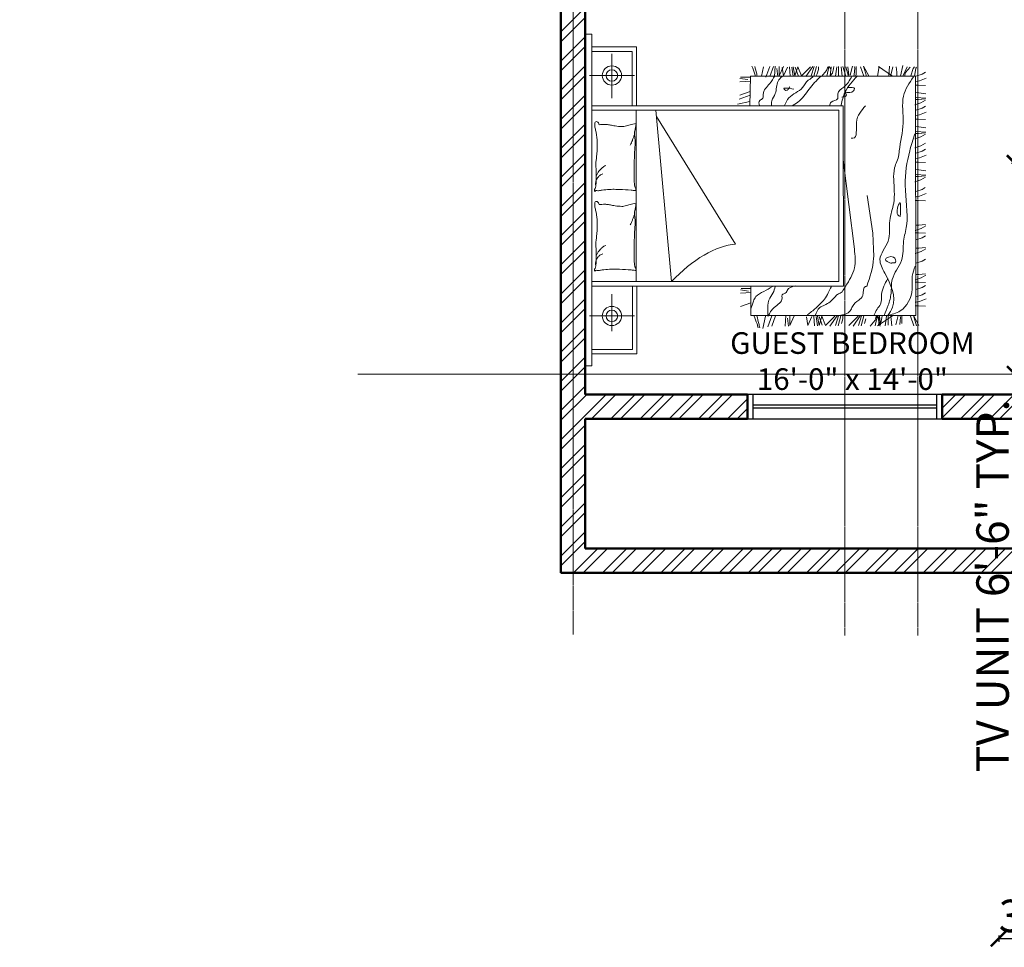
# Model space of a CAD drawing. Units: inches. Extents: x 261 to 2725, y 291 to 1454.
# Tile 17 of 35: x 1043 to 1407, y 301 to 644. Entities that reach past the tile are written whole.
import ezdxf

# ---------------------------------------------------------------- set-up
doc = ezdxf.new("R2010")
doc.units = ezdxf.units.IN
doc.linetypes.add('CENTER', pattern=[2, 1.25, -0.25, 0.25, -0.25])
for name, color, linetype, lineweight in [('A-ANNO-DIMS', 136, 'Continuous', 18), ('A-AREA-IDEN', 18, 'Continuous', 18), ('A-DOOR', 160, 'Continuous', 25), ('A-FURN', 30, 'Continuous', 18), ('A-GLAZ', 150, 'Continuous', 25), ('A-GRID', 251, 'CENTER', 13), ('A-WALL', 222, 'Continuous', 50), ('A-WALL-PATT', 243, 'Continuous', 13)]:
    doc.layers.add(name, color=color, linetype=linetype, lineweight=lineweight)
doc.styles.get("Standard").update_dxf_attribs({"font": 'arial.ttf'})
doc.dimstyles.new('ISO-25', dxfattribs={"dimtxt": 12, "dimasz": 6, "dimexe": 1.25, "dimexo": 0.625, "dimtad": 1, "dimdec": 0, "dimlunit": 3, "dimtxsty": 'Standard', "dimblk": 'ARCHTICK', "dimcen": 2.5, "dimadec": 0, "dimazin": 0, "dimtfac": 1, "dimtdec": 0, "dimtmove": 0, "dimatfit": 3, "dimfxl": 1, "dimfxlon": 1, "dimarcsym": 0})

# ---------------------------------------------------------------- blocks, each defined once
blk = doc.blocks.new('*U6')
for p, q in [((-36, 0), (-36, 6)), ((0, 0), (0, 6))]:
    blk.add_line(p, q)
blk.add_lwpolyline([(0, 0), (0, -36), (-1.75, -36), (-1.75, 0)], close=True)
blk.add_arc((0, 0), 36, 180, 270)
blk = doc.blocks.new('A$C2B723114')
for p, q in [((0, 2.9047), (2.8274, 2.9047)), ((0, 2.8487), (0, 2.9047)), ((0.4243, 2.8697), (0.4243, 2.4855)), ((2.4742, 2.8697), (2.4742, 2.4855)), ((2.8274, 2.9047), (2.8274, 2.8487)), ((2.8274, 2.8487), (0, 2.8487)), ((0.1012, 2.4649), (0.1012, 2.849)), ((0.1396, 2.5033), (0.1396, 2.849)), ((0.6794, 0.7051), (0.6794, 2.8509)), ((0.7187, 0.7435), (0.7187, 2.8509)), ((2.1776, 2.8509), (2.1776, 0.7454)), ((2.216, 2.8509), (2.216, 0.707)), ((2.6798, 2.5052), (2.6798, 2.8509)), ((2.7182, 2.4668), (2.7182, 2.8509)), ((0.6087, 2.6776), (0.295, 2.6776)), ((2.6586, 2.6776), (2.2821, 2.6776)), ((1.3789, 2.4999), (1.3598, 2.5761)), ((2.0593, 2.4999), (2.0402, 2.5761)), ((0.6794, 2.4649), (0.1012, 2.4649)), ((0.6766, 2.5033), (0.1396, 2.5033)), ((0.7191, 2.47), (2.1778, 2.4719)), ((1.3858, 2.4723), (1.3789, 2.4999)), ((2.0662, 2.4723), (2.0593, 2.4999)), ((2.2188, 2.5052), (2.6798, 2.5052)), ((2.2188, 2.4668), (2.7182, 2.4668)), ((2.1771, 2.3036), (0.718, 2.1685)), ((1.0365, 1.6233), (2.1246, 2.2989)), ((2.2287, 1.6076), (2.2523, 1.5035)), ((0.5047, 1.5819), (0.5353, 1.4945)), ((0.6174, 1.5819), (0.6232, 1.4916)), ((0.6467, 1.5819), (0.6369, 1.5137)), ((0.6571, 1.4945), (0.6571, 1.5765)), ((2.2726, 1.593), (2.3061, 1.5007)), ((2.3067, 1.5881), (2.3373, 1.5007)), ((2.4194, 1.5881), (2.4251, 1.4979)), ((2.4487, 1.5881), (2.4389, 1.5199)), ((2.4591, 1.5007), (2.4591, 1.5828)), ((0.4269, 0.0884), (0.4269, 1.4945)), ((0.4269, 1.4945), (0.6794, 1.4945)), ((2.4685, 1.4964), (2.216, 1.5022)), ((2.4685, 1.4964), (2.4685, 0.0903)), ((0.3172, 1.3923), (0.4213, 1.3687)), ((0.3318, 1.3485), (0.4241, 1.3149)), ((2.4596, 1.3659), (2.552, 1.3324)), ((2.4685, 1.4044), (2.5491, 1.3861)), ((0.3367, 1.3143), (0.4241, 1.2838)), ((2.4645, 1.3318), (2.552, 1.3012)), ((2.4645, 1.2928), (2.5548, 1.2871)), ((2.4645, 1.2635), (2.5328, 1.2733)), ((0.3367, 1.2016), (0.427, 1.1959)), ((0.3367, 1.1724), (0.405, 1.1821)), ((2.4699, 1.2531), (2.552, 1.2163)), ((2.552, 1.2531), (2.4699, 1.2531)), ((2.5435, 1.2276), (2.4699, 1.2163)), ((2.4699, 1.2163), (2.5463, 1.1823)), ((0.4241, 1.162), (0.3421, 1.162)), ((0.3421, 1.162), (0.4241, 1.1252)), ((2.5491, 1.1654), (2.467, 1.1597)), ((2.5463, 1.1455), (2.467, 1.1342)), ((2.5491, 1.1342), (2.4699, 1.1201)), ((2.4699, 1.1201), (2.5491, 1.0946)), ((2.5491, 1.0946), (2.4699, 1.0635)), ((2.5463, 1.1172), (2.4727, 1.0918)), ((0.4157, 1.0206), (0.3421, 1.0093)), ((0.3421, 1.0093), (0.4185, 0.9754)), ((2.4642, 1.0267), (2.552, 0.9644)), ((2.4699, 1.0635), (2.5491, 0.9842)), ((0.4213, 0.9584), (0.3392, 0.9527)), ((0.4185, 0.9386), (0.3392, 0.9272)), ((0.4213, 0.9272), (0.3421, 0.9131)), ((2.4642, 0.9389), (2.4869, 0.9276)), ((2.467, 0.9559), (2.552, 0.9333)), ((2.4699, 0.9785), (2.552, 0.9531)), ((2.4869, 0.9276), (2.5265, 0.9163)), ((0.3421, 0.9131), (0.4213, 0.8876)), ((0.4213, 0.8876), (0.3421, 0.8565)), ((0.3421, 0.8565), (0.4213, 0.7772)), ((0.4185, 0.9103), (0.3449, 0.8848)), ((2.4642, 0.8908), (2.5152, 0.8483)), ((2.467, 0.8455), (2.5208, 0.8342)), ((2.5152, 0.8483), (2.5491, 0.837)), ((2.5265, 0.9163), (2.5491, 0.9163)), ((0.3364, 0.8197), (0.4241, 0.7574)), ((0.3421, 0.7716), (0.4241, 0.7461)), ((2.5491, 0.7606), (2.467, 0.7719)), ((2.4699, 0.8172), (2.4925, 0.7974)), ((2.5491, 0.8087), (2.4699, 0.8172)), ((2.4925, 0.7974), (2.535, 0.7889)), ((2.5208, 0.8342), (2.552, 0.8285)), ((2.552, 0.8285), (2.5293, 0.8087)), ((2.535, 0.7889), (2.552, 0.7861)), ((0.3392, 0.7489), (0.4241, 0.7263)), ((0.359, 0.7206), (0.3987, 0.7093)), ((0.3987, 0.7093), (0.4213, 0.7093)), ((2.216, 0.707), (0.6794, 0.7051)), ((2.1776, 0.7454), (0.7187, 0.7435)), ((0.9938, 0.6115), (1.7555, 0.7064)), ((2.5491, 0.6842), (2.4642, 0.6615)), ((2.4727, 0.7464), (2.467, 0.7408)), ((2.467, 0.7153), (2.5491, 0.7238)), ((2.552, 0.7096), (2.467, 0.6842)), ((2.552, 0.7464), (2.4727, 0.7464)), ((0.3364, 0.6233), (0.4241, 0.561)), ((0.3421, 0.6601), (0.4213, 0.5808)), ((2.4642, 0.6191), (2.4784, 0.6134)), ((2.467, 0.5993), (2.4869, 0.5964)), ((2.5491, 0.6672), (2.4755, 0.6587)), ((2.4755, 0.6474), (2.5548, 0.6276)), ((2.4784, 0.6134), (2.5406, 0.6077)), ((2.4869, 0.5964), (2.552, 0.5964)), ((2.5406, 0.6077), (2.552, 0.6134)), ((0.3392, 0.5525), (0.4241, 0.5299)), ((0.3421, 0.5752), (0.4241, 0.5497)), ((0.359, 0.5242), (0.3987, 0.5129)), ((2.467, 0.5313), (2.5491, 0.5596)), ((2.467, 0.5087), (2.5548, 0.5342)), ((2.5548, 0.5342), (2.4699, 0.4889)), ((0.3364, 0.4785), (0.3874, 0.436)), ((0.3392, 0.4332), (0.393, 0.4219)), ((0.3874, 0.436), (0.4213, 0.4247)), ((0.393, 0.4219), (0.4241, 0.4162)), ((1.1305, 0.4537), (0.9938, 0.448)), ((1.4523, 0.5021), (1.1305, 0.4537)), ((0.4213, 0.415), (0.3364, 0.3923)), ((0.4241, 0.2868), (0.3392, 0.415)), ((0.4213, 0.3377), (0.3392, 0.3491)), ((0.3421, 0.4049), (0.3647, 0.3851)), ((0.4213, 0.3964), (0.3421, 0.4049)), ((0.4213, 0.398), (0.3477, 0.3895)), ((0.3647, 0.3851), (0.4072, 0.3766)), ((0.4241, 0.4162), (0.4015, 0.3964)), ((0.4072, 0.3766), (0.4241, 0.3738)), ((2.467, 0.4133), (2.552, 0.4019)), ((2.467, 0.2879), (2.552, 0.4076)), ((0.3392, 0.2925), (0.4213, 0.3009)), ((0.4241, 0.3236), (0.3449, 0.3236)), ((0.3477, 0.2571), (0.427, 0.2373)), ((2.4642, 0.3049), (2.5491, 0.2851)), ((2.467, 0.319), (2.5548, 0.3134)), ((2.501, 0.2491), (2.5491, 0.2547)), ((0.3506, 0.2231), (0.4128, 0.2175)), ((0.359, 0.2061), (0.4241, 0.2061)), ((0.4128, 0.2175), (0.4241, 0.2231)), ((2.467, 0.2179), (2.5605, 0.1981)), ((2.467, 0.1981), (2.5491, 0.1613)), ((2.467, 0.184), (2.4982, 0.1755)), ((2.4699, 0.2491), (2.501, 0.2491)), ((2.4982, 0.1755), (2.5463, 0.1359)), ((0.3392, 0.1042), (0.4213, 0.1325)), ((0.3392, 0.0815), (0.427, 0.107)), ((0.427, 0.107), (0.3421, 0.0617)), ((2.4685, 0.0903), (0.4269, 0.0884)), ((0.5106, 0.094), (0.5106, 0.0657)), ((0.5417, 0.094), (0.5474, 0.0572)), ((0.587, 0.0884), (0.604, 0.0346)), ((0.6512, 0.0884), (0.6682, 0.0346)), ((0.713, 0.094), (0.713, 0.0657)), ((0.7334, 0.0943), (0.7503, 0.0434)), ((0.7786, 0.0915), (0.7786, 0.0632)), ((0.8739, 0.0884), (0.8908, 0.0346)), ((0.956, 0.0943), (0.973, 0.0434)), ((1.0013, 0.0915), (1.0013, 0.0632)), ((1.072, 0.0884), (1.089, 0.0346)), ((1.1338, 0.094), (1.1338, 0.0657)), ((1.1542, 0.0943), (1.1712, 0.0434)), ((1.1995, 0.0915), (1.1995, 0.0632)), ((1.4088, 0.094), (1.4088, 0.0657)), ((1.44, 0.094), (1.4456, 0.0572)), ((1.4853, 0.0884), (1.5023, 0.0346)), ((1.5674, 0.0962), (1.5844, 0.0453)), ((1.6127, 0.0934), (1.6127, 0.0651)), ((1.6297, 0.0849), (1.624, 0.0028)), ((1.6721, 0.0877), (1.6693, 0.0623)), ((1.7344, 0.0934), (1.7344, 0.0651)), ((1.7655, 0.0934), (1.7712, 0.0566)), ((1.8108, 0.0877), (1.8278, 0.034)), ((1.8568, 0.0962), (1.8738, 0.0453)), ((1.9342, 0.0962), (1.9512, 0.0453)), ((1.9795, 0.0934), (1.9795, 0.0651)), ((1.9965, 0.0849), (1.9908, 0.0028)), ((2.039, 0.0877), (2.0361, 0.0623)), ((2.1012, 0.0934), (2.1012, 0.0651)), ((2.1324, 0.0934), (2.138, 0.0566)), ((2.1777, 0.0877), (2.1946, 0.034)), ((2.2236, 0.0962), (2.2406, 0.0453)), ((2.2689, 0.0934), (2.2689, 0.0651)), ((2.2859, 0.0849), (2.2802, 0.0028)), ((2.3284, 0.0877), (2.3255, 0.0623)), ((2.3906, 0.0934), (2.3906, 0.0651)), ((2.4218, 0.0934), (2.4274, 0.0566)), ((2.4642, 0.0991), (2.5378, 0.0877)), ((2.467, 0.0877), (2.484, 0.034)), ((2.4699, 0.1302), (2.535, 0.1104)), ((2.535, 0.1104), (2.5491, 0.0991)), ((2.5378, 0.0877), (2.5463, 0.0821)), ((0.5106, 0.0657), (0.5077, 0.0063)), ((0.5474, 0.0572), (0.57, 0.0006)), ((0.604, 0.0346), (0.621, 0.0063)), ((0.6682, 0.0346), (0.6851, 0.0063)), ((0.713, 0.0657), (0.7101, 0.0063)), ((0.7503, 0.0434), (0.773, 0.0037)), ((0.7786, 0.0632), (0.7843, 0.0066)), ((0.8908, 0.0346), (0.9078, 0.0063)), ((0.973, 0.0434), (0.9957, 0.0037)), ((1.0013, 0.0632), (1.007, 0.0066)), ((1.089, 0.0346), (1.106, 0.0063)), ((1.1338, 0.0657), (1.131, 0.0063)), ((1.1712, 0.0434), (1.1939, 0.0037)), ((1.1995, 0.0632), (1.2052, 0.0066)), ((1.4088, 0.0657), (1.406, 0.0063)), ((1.4456, 0.0572), (1.4683, 0.0006)), ((1.5023, 0.0346), (1.5192, 0.0082)), ((1.5844, 0.0453), (1.607, 0.0057)), ((1.6127, 0.0651), (1.6184, 0.0085)), ((1.6693, 0.0623), (1.6608, 0.0028)), ((1.7344, 0.0651), (1.7316, 0.0057)), ((1.7712, 0.0566), (1.7938, 0)), ((1.8278, 0.034), (1.8448, 0.0057)), ((1.8738, 0.0453), (1.8964, 0.0057)), ((1.9512, 0.0453), (1.9739, 0.0057)), ((1.9795, 0.0651), (1.9852, 0.0085)), ((2.0361, 0.0623), (2.0276, 0.0028)), ((2.1012, 0.0651), (2.0984, 0.0057)), ((2.138, 0.0566), (2.1607, 0)), ((2.1946, 0.034), (2.2116, 0.0057)), ((2.2406, 0.0453), (2.2632, 0.0057)), ((2.2689, 0.0651), (2.2746, 0.0085)), ((2.3255, 0.0623), (2.317, 0.0028)), ((2.3906, 0.0651), (2.3878, 0.0057)), ((2.4274, 0.0566), (2.4501, 0)), ((2.484, 0.034), (2.501, 0.0057))]:
    blk.add_line(p, q)
for centre, radius in [((0.4243, 2.6776), 0.0821), ((0.4243, 2.6776), 0.0493), ((2.4742, 2.6776), 0.0821), ((2.4742, 2.6776), 0.0493)]:
    blk.add_circle(centre, radius)
for centre, radius, start, end in [((0.8078, 2.821), 0.00214, 160.43603, 281.89306), ((0.8088, 2.8207), 0.00315, 111.7883, 160.43603), ((0.8162, 2.8021), 0.0232, 94.30254, 111.7883), ((0.8091, 2.8151), 0.00394, 21.9904, 101.89306), ((0.8409, 2.7949), 0.0302, 158.57902, 188.13348), ((1.0356, 2.8227), 0.2268, 188.13348, 192.10946), ((0.7994, 2.8112), 0.0144, 338.57902, 21.9904), ((0.635, 2.7368), 0.1829, 7.6809, 12.10946), ((0.8165, 2.7987), 0.0266, 59.34875, 94.30254), ((0.8554, 2.8643), 0.0497, 239.34875, 264.74081), ((0.9202, 3.5684), 0.7568, 264.74081, 268.09211), ((0.8679, 2.7254), 0.0915, 74.06476, 94.21588), ((0.8679, 2.7254), 0.0915, 53.91364, 74.06476), ((0.9409, 4.189), 1.3777, 268.09211, 270.57574), ((0.8679, 2.7254), 0.0915, 36.17665, 53.91364), ((0.86, 2.6097), 0.2158, 62.76041, 69.13972), ((0.8679, 2.7254), 0.0915, 18.43965, 36.17665), ((0.9466, 3.6164), 0.8051, 270.57574, 274.80185), ((0.9263, 2.7386), 0.0708, 51.61143, 62.76041), ((0.7461, 2.511), 0.3611, 46.18849, 51.61143), ((0.8523, 2.6218), 0.2076, 39.03494, 46.18849), ((1.0364, 2.548), 0.2671, 87.46141, 94.80185), ((1.042, 2.6745), 0.1405, 79.81012, 87.46141), ((1.1532, 3.2931), 0.488, 259.81012, 263.9133), ((1.204, 3.7695), 0.9671, 263.9133, 270), ((1.204, 3.4318), 0.6294, 270, 277.54685), ((1.2573, 3.0292), 0.2233, 277.54685, 285.74398), ((1.3941, 2.5438), 0.281, 98.43719, 105.74398), ((1.3747, 2.6748), 0.1486, 90, 98.43719), ((1.3713, 2.8186), 0.0315, 274.40021, 333.41948), ((0.923, 2.7382), 0.4535, 0, 6.23236), ((1.3747, 2.74), 0.0833, 78.72762, 90), ((1.3886, 2.8099), 0.0121, 333.41948, 78.72762), ((1.4882, 2.821), 0.00214, 160.43603, 281.89306), ((1.4892, 2.8207), 0.00315, 111.7883, 160.43603), ((1.4966, 2.8021), 0.0232, 94.30254, 111.7883), ((1.4895, 2.8151), 0.00394, 21.9904, 101.89306), ((1.5213, 2.7949), 0.0302, 158.57902, 188.13348), ((1.716, 2.8227), 0.2268, 188.13348, 192.10946), ((1.4798, 2.8112), 0.0144, 338.57902, 21.9904), ((1.3154, 2.7368), 0.1829, 7.6809, 12.10946), ((1.4969, 2.7987), 0.0266, 59.34875, 94.30254), ((1.5358, 2.8643), 0.0497, 239.34875, 264.74081), ((1.6006, 3.5684), 0.7568, 264.74081, 268.09211), ((1.5483, 2.7254), 0.0915, 74.06476, 94.21588), ((1.5483, 2.7254), 0.0915, 53.91364, 74.06476), ((1.6213, 4.189), 1.3777, 268.09211, 270.57574), ((1.5483, 2.7254), 0.0915, 36.17665, 53.91364), ((1.5404, 2.6097), 0.2158, 62.76041, 69.13972), ((1.5483, 2.7254), 0.0915, 18.43965, 36.17665), ((1.627, 3.6164), 0.8051, 270.57574, 274.80185), ((1.6067, 2.7386), 0.0708, 51.61143, 62.76041), ((1.4265, 2.511), 0.3611, 46.18849, 51.61143), ((1.5327, 2.6218), 0.2076, 39.03494, 46.18849), ((1.7168, 2.548), 0.2671, 87.46141, 94.80185), ((1.7224, 2.6745), 0.1405, 79.81012, 87.46141), ((1.8336, 3.2931), 0.488, 259.81012, 263.9133), ((1.8844, 3.7695), 0.9671, 263.9133, 270), ((1.8844, 3.4318), 0.6294, 270, 277.54685), ((1.9377, 3.0292), 0.2233, 277.54685, 285.74398), ((2.0745, 2.5438), 0.281, 98.43719, 105.74398), ((2.0551, 2.6748), 0.1486, 90, 98.43719), ((2.0517, 2.8186), 0.0315, 274.40021, 333.41948), ((1.6034, 2.7382), 0.4535, 0, 6.23236), ((2.0551, 2.74), 0.0833, 78.72762, 90), ((2.069, 2.8099), 0.0121, 333.41948, 78.72762), ((-0.0181, 2.6487), 0.8418, 3.36875, 7.6809), ((0.1976, 2.6614), 0.6258, 358.36691, 3.36875), ((0.9783, 2.7239), 0.0455, 28.31676, 39.03494), ((0.8558, 2.6579), 0.1846, 23.00277, 28.31676), ((0.5722, 2.8434), 0.8132, 347.80162, 350.31563), ((1.1884, 2.7382), 0.1881, 350.31563, 0), ((0.6623, 2.6487), 0.8418, 3.36875, 7.6809), ((0.878, 2.6614), 0.6258, 358.36691, 3.36875), ((1.6587, 2.7239), 0.0455, 28.31676, 39.03494), ((1.5362, 2.6579), 0.1846, 23.00277, 28.31676), ((1.2526, 2.8434), 0.8132, 347.80162, 350.31563), ((1.8688, 2.7382), 0.1881, 350.31563, 0), ((-11.7321, 3.2823), 12.5718, 356.49514, 356.94504), ((-0.4351, 2.6794), 1.2587, 356.94504, 358.36691), ((1.9648, 2.5659), 0.6074, 171.99495, 177.33512), ((1.6528, 2.6098), 0.2924, 167.80162, 171.99495), ((-11.0517, 3.2823), 12.5718, 356.49514, 356.94504), ((0.2453, 2.6794), 1.2587, 356.94504, 358.36691), ((2.6452, 2.5659), 0.6074, 171.99495, 177.33512), ((2.3332, 2.6098), 0.2924, 167.80162, 171.99495), ((1.4917, 3.1364), 0.681, 244.68893, 246.51559), ((1.4204, 2.5912), 0.0624, 177.33512, 194.04519), ((2.1721, 3.1364), 0.681, 244.68893, 246.51559), ((2.1008, 2.5912), 0.0624, 177.33512, 194.04519), ((0.8298, 2.4774), 0.0178, 170.00164, 196.69777), ((0.5206, 2.5319), 0.2961, 350.00164, 356.49514), ((0.8139, 2.4726), 0.00122, 196.69777, 277.12039), ((0.8041, 2.5514), 0.0807, 277.12039, 286.22115), ((0.8068, 2.5419), 0.0707, 286.22115, 297.28412), ((0.8584, 2.4419), 0.0418, 102.86904, 117.28412), ((0.879, 2.3515), 0.1345, 93.57397, 102.86904), ((0.9376, 1.4146), 1.0732, 90.28654, 93.57397), ((0.9586, -2.7845), 5.2724, 89.02962, 90.28654), ((0.9954, -0.6123), 3.0999, 87.39037, 89.02962), ((1.0854, 1.364), 1.1216, 85.38242, 87.39037), ((1.28, 3.7729), 1.2952, 265.38242, 267.25094), ((1.228, 2.691), 0.2121, 267.25094, 281.55856), ((1.4917, 3.1364), 0.681, 246.51559, 248.34226), ((1.4917, 3.1364), 0.681, 248.34226, 250.57202), ((1.4917, 3.1364), 0.681, 250.57202, 252.80178), ((1.2975, 2.3514), 0.1345, 83.56595, 101.55856), ((1.3002, 2.3754), 0.1104, 72.61359, 83.56595), ((1.3965, 2.6828), 0.2118, 252.61359, 260.5159), ((1.4027, 2.7202), 0.2496, 260.5159, 265.91706), ((1.385, 2.4721), 0.000845, 265.91706, 14.04494), ((1.5102, 2.4774), 0.0178, 170.00164, 196.69777), ((1.201, 2.5319), 0.2961, 350.00164, 356.49514), ((1.4943, 2.4726), 0.00122, 196.69777, 277.12039), ((1.4845, 2.5514), 0.0807, 277.12039, 286.22115), ((1.4872, 2.5419), 0.0707, 286.22115, 297.28412), ((1.5388, 2.4419), 0.0418, 102.86904, 117.28412), ((1.5594, 2.3515), 0.1345, 93.57397, 102.86904), ((1.618, 1.4146), 1.0732, 90.28654, 93.57397), ((1.639, -2.7845), 5.2724, 89.02962, 90.28654), ((1.6758, -0.6123), 3.0999, 87.39037, 89.02962), ((1.7658, 1.364), 1.1216, 85.38242, 87.39037), ((1.9604, 3.7729), 1.2952, 265.38242, 267.25094), ((1.9084, 2.691), 0.2121, 267.25094, 281.55856), ((2.1721, 3.1364), 0.681, 246.51559, 248.34226), ((2.1721, 3.1364), 0.681, 248.34226, 250.57202), ((2.1721, 3.1364), 0.681, 250.57202, 252.80178), ((1.9779, 2.3514), 0.1345, 83.56595, 101.55856), ((1.9806, 2.3754), 0.1104, 72.61359, 83.56595), ((2.0769, 2.6828), 0.2118, 252.61359, 260.5159), ((2.0831, 2.7202), 0.2496, 260.5159, 265.91706), ((2.0654, 2.4721), 0.000845, 265.91706, 14.04494)]:
    blk.add_arc(centre, radius, start, end)
blk.add_ellipse((0.4962, 1.9132), major_axis=(0.4887, -0.4605), ratio=0.503305, start_param=0.491272, end_param=1.591113)
for points, knots in [([(0.427, 1.4678), (0.4036, 1.4582), (0.3693, 1.4441), (0.3335, 1.4344), (0.3221, 1.4313)], [0, 0, 0, 0, 98.452083, 144.639601, 144.639601, 144.639601, 144.639601]), ([(0.4241, 1.4423), (0.4031, 1.437), (0.3691, 1.4284), (0.3351, 1.4199), (0.3221, 1.4167)], [0, 0, 0, 0, 84.638756, 136.955563, 136.955563, 136.955563, 136.955563]), ([(0.6768, 1.3104), (0.6615, 1.3339), (0.6315, 1.3797), (0.604, 1.4501), (0.5417, 1.4748), (0.5064, 1.4871), (0.4848, 1.4945)], [0, 0, 0, 0, 110.980521, 216.571322, 273.316778, 363.252298, 363.252298, 363.252298, 363.252298]), ([(2.2145, 1.4211), (2.233, 1.4246), (2.2636, 1.4303), (2.2761, 1.3837), (2.3429, 1.3967), (2.3949, 1.3342), (2.4474, 1.3031), (2.4698, 1.2898)], [0, 0, 0, 0, 61.886907, 102.717887, 145.699352, 284.082577, 386.765171, 386.765171, 386.765171, 386.765171]), ([(2.5548, 1.4853), (2.5314, 1.4757), (2.5031, 1.4641), (2.4737, 1.4555), (2.4685, 1.454)], [0, 0, 0, 0, 98.452083, 119.481049, 119.481049, 119.481049, 119.481049]), ([(2.552, 1.4598), (2.5309, 1.4545), (2.5031, 1.4475), (2.4753, 1.4406), (2.4685, 1.4389)], [0, 0, 0, 0, 84.638756, 111.94623, 111.94623, 111.94623, 111.94623]), ([(0.6768, 1.286), (0.6567, 1.2911), (0.6145, 1.3017), (0.5543, 1.3533), (0.4816, 1.349), (0.4362, 1.3493), (0.4233, 1.3493)], [0, 0, 0, 0, 80.250278, 168.388677, 295.908361, 346.663112, 346.663112, 346.663112, 346.663112]), ([(0.4233, 1.3445), (0.4367, 1.3385), (0.464, 1.3264), (0.5129, 1.2848), (0.5456, 1.2161), (0.6131, 1.2349), (0.6142, 1.1913), (0.6642, 1.1806), (0.674, 1.144), (0.6817, 1.1154)], [0, 0, 0, 0, 56.745495, 115.23739, 254.956954, 286.678662, 337.828324, 366.201072, 468.500395, 468.500395, 468.500395, 468.500395]), ([(2.2145, 1.319), (2.2295, 1.319), (2.2678, 1.3192), (2.3288, 1.2705), (2.4143, 1.279), (2.4535, 1.2403), (2.4662, 1.2278)], [0, 0, 0, 0, 57.155505, 146.33427, 287.936209, 355.396728, 355.396728, 355.396728, 355.396728]), ([(2.2182, 1.2059), (2.2419, 1.1958), (2.3116, 1.1659), (2.342, 1.0552), (2.4266, 1.0223), (2.4474, 0.9811), (2.462, 0.9684), (2.4698, 0.9616)], [0, 0, 0, 0, 97.73655, 287.59661, 389.176293, 423.403759, 463.679181, 463.679181, 463.679181, 463.679181]), ([(2.3573, 1.127), (2.3656, 1.1759), (2.3758, 1.2352), (2.3371, 1.1853), (2.3602, 1.1713), (2.3768, 1.1612)], [0, 0, 0, 0, 107.853607, 130.728419, 189.220329, 189.220329, 189.220329, 189.220329]), ([(2.2145, 1.1476), (2.2246, 1.1286), (2.2575, 1.0666), (2.3612, 1.0009), (2.431, 0.9336), (2.4662, 0.8996)], [0, 0, 0, 0, 83.02987, 271.460712, 463.033803, 463.033803, 463.033803, 463.033803]), ([(0.6817, 0.8034), (0.6673, 0.8119), (0.6341, 0.8315), (0.5785, 0.8518), (0.5349, 0.8973), (0.4828, 0.9461), (0.4518, 0.9879), (0.4331, 1.013)], [0, 0, 0, 0, 65.318952, 150.437229, 226.833166, 307.58338, 429.454095, 429.454095, 429.454095, 429.454095]), ([(0.4282, 0.9448), (0.4547, 0.9353), (0.496, 0.9206), (0.5223, 0.8436), (0.5628, 0.7946), (0.6113, 0.7575), (0.6214, 0.7173), (0.6539, 0.7022), (0.672, 0.6897), (0.6768, 0.6864)], [0, 0, 0, 0, 102.299436, 159.044876, 303.717955, 348.579152, 391.138254, 454.581655, 477.456496, 477.456496, 477.456496, 477.456496]), ([(2.2145, 0.823), (2.227, 0.8201), (2.261, 0.8121), (2.261, 0.7401), (2.3352, 0.7659), (2.379, 0.6836), (2.4336, 0.6521), (2.4662, 0.6334)], [0, 0, 0, 0, 46.747668, 127.438174, 179.649794, 280.561838, 429.605131, 429.605131, 429.605131, 429.605131]), ([(0.4282, 0.74), (0.4347, 0.7029), (0.444, 0.6496), (0.5194, 0.6274), (0.555, 0.5807), (0.5975, 0.5243), (0.6789, 0.5415), (0.677, 0.5095), (0.6768, 0.5061)], [0, 0, 0, 0, 130.791737, 187.537266, 286.231946, 353.673191, 460.023761, 472.712403, 472.712403, 472.712403, 472.712403]), ([(0.6768, 0.6864), (0.7275, 0.655), (0.8251, 0.5944), (0.9391, 0.606), (0.9938, 0.6115)], [0, 0, 0, 0, 225.995823, 434.686543, 434.686543, 434.686543, 434.686543]), ([(2.2218, 0.7246), (2.2595, 0.716), (2.3548, 0.6945), (2.4265, 0.6268), (2.4698, 0.586)], [0, 0, 0, 0, 148.665024, 375.555892, 375.555892, 375.555892, 375.555892]), ([(2.3719, 0.6737), (2.3738, 0.6431), (2.3772, 0.5878), (2.3146, 0.6382), (2.3401, 0.7015), (2.2971, 0.6649), (2.2923, 0.6965), (2.289, 0.7176)], [0, 0, 0, 0, 83.446591, 150.887818, 201.642461, 230.015204, 286.760644, 286.760644, 286.760644, 286.760644]), ([(2.2145, 0.5167), (2.1764, 0.5522), (2.1051, 0.6184), (1.9357, 0.5803), (1.9385, 0.6342), (1.9388, 0.6395)], [0, 0, 0, 0, 208.073343, 389.01094, 409.01094, 409.01094, 409.01094, 409.01094]), ([(0.6768, 0.5061), (0.7554, 0.4794), (0.8591, 0.4442), (0.9675, 0.4473), (0.9938, 0.448)], [0, 0, 0, 0, 319.374611, 421.61723, 421.61723, 421.61723, 421.61723]), ([(0.4331, 0.4427), (0.4498, 0.4356), (0.4827, 0.4216), (0.5314, 0.3759), (0.632, 0.3884), (0.6996, 0.3513), (0.7423, 0.3278)], [0, 0, 0, 0, 70.931849, 139.556414, 248.154027, 434.709995, 434.709995, 434.709995, 434.709995]), ([(2.4625, 0.1088), (2.4095, 0.1438), (2.2904, 0.2226), (2.0623, 0.1771), (1.9006, 0.2246), (1.7699, 0.2337), (1.6941, 0.2766), (1.5528, 0.2786), (1.4005, 0.2587), (1.2324, 0.3267), (1.059, 0.2939), (0.9218, 0.426), (0.7359, 0.3204), (0.5586, 0.2391), (0.4502, 0.3116), (0.427, 0.3272)], [0, 0, 0, 0, 239.874704, 538.942419, 850.40885, 893.390315, 1047.998294, 1176.505142, 1437.500972, 1637.333004, 1864.324391, 2089.058767, 2248.736533, 2637.953392, 2744.252142, 2744.252142, 2744.252142, 2744.252142]), ([(1.9771, 0.0962), (1.9286, 0.1117), (1.7864, 0.157), (1.5223, 0.1992), (1.2611, 0.141), (1.0527, 0.2023), (0.8859, 0.1885), (0.76, 0.3042), (0.6211, 0.292), (0.5187, 0.3203), (0.4572, 0.3456), (0.4282, 0.3575)], [0, 0, 0, 0, 198.710624, 582.73994, 1031.873213, 1206.082894, 1423.278209, 1655.952104, 1808.744089, 1945.69963, 2068.229211, 2068.229211, 2068.229211, 2068.229211]), ([(0.8718, 0.2941), (0.8821, 0.3221), (0.9041, 0.3814), (0.9523, 0.2773), (0.8733, 0.2454), (0.8757, 0.2798), (0.8766, 0.2941)], [0, 0, 0, 0, 82.720021, 175.094899, 237.579423, 282.440623, 282.440623, 282.440623, 282.440623]), ([(0.8474, 0.0943), (0.82, 0.1047), (0.757, 0.1287), (0.6201, 0.1029), (0.4623, 0.1837), (0.4372, 0.2936), (0.4282, 0.3331)], [0, 0, 0, 0, 112.422038, 258.341957, 533.791494, 688.286079, 688.286079, 688.286079, 688.286079]), ([(1.2715, 0.221), (1.3344, 0.2172), (1.4529, 0.21), (1.2971, 0.2665), (1.2756, 0.2284), (1.2715, 0.221)], [0, 0, 0, 0, 150.888188, 283.977876, 315.699589, 315.699589, 315.699589, 315.699589])]:
    blk.add_open_spline(points, degree=3, knots=knots)
blk = doc.blocks.new('WIN-72')
for p, q in [((955.45, 950.47), (946.45, 950.47)), ((950.45, 950.47), (950.45, 882.47)), ((951.45, 882.47), (951.45, 950.47)), ((946.45, 882.47), (955.45, 882.47))]:
    blk.add_line(p, q)
blk.add_lwpolyline([(955.45, 880.47), (955.45, 952.47), (946.45, 952.47), (946.45, 880.47)], close=True)
blk = doc.blocks.new('_ArchTick')
at = {"color": 0, "linetype": 'ByBlock', "const_width": 0.15}
blk.add_lwpolyline([(-0.5, -0.5), (0.5, 0.5)], dxfattribs=at)
blk = doc.blocks.new('*D43')
at = {"layer": 'A-ANNO-DIMS', "color": 0, "lineweight": -2, "ltscale": 0.07, "transparency": 16777216}
for p, q in [((1412.05, 590.97), (1409.8, 590.97)), ((1411.05, 590.97), (1411.05, 512.97)), ((1412.05, 512.97), (1409.8, 512.97)), ((1411.05, 512.97), (1411.05, 362.42))]:
    blk.add_line(p, q, dxfattribs=at)
at = {"layer": 'Defpoints', "color": 0, "ltscale": 0.07, "transparency": 16777216}
for p in [(1422.75, 590.97), (1411.05, 512.97), (1422.75, 512.97)]:
    blk.add_point(p, dxfattribs=at)
at = {"layer": 'A-ANNO-DIMS', "color": 0, "lineweight": -2, "ltscale": 0.07, "transparency": 16777216, "xscale": 6, "yscale": 6, "zscale": 6}
for p, rotation in [((1411.05, 590.97), 90), ((1411.05, 512.97), 270)]:
    blk.add_blockref('_ArchTick', p, dxfattribs=dict(at, rotation=rotation))
at = {"layer": 'A-ANNO-DIMS', "color": 0, "ltscale": 0.07, "transparency": 16777216, "insert": (1404.29, 434.7), "char_height": 12, "attachment_point": 5, "rotation": 90}
blk.add_mtext('TV UNIT 6\'-6" TYP.', dxfattribs=at)
blk = doc.blocks.new('*D82')
at = {"layer": 'A-ANNO-DIMS', "color": 0, "lineweight": -2, "ltscale": 0.07, "transparency": 16777216}
for p, q in [((2600.96, 679.47), (2603.21, 679.47)), ((2601.96, 517.47), (2601.96, 679.47)), ((2600.96, 517.47), (2603.21, 517.47))]:
    blk.add_line(p, q, dxfattribs=at)
at = {"layer": 'Defpoints', "color": 0, "ltscale": 0.07, "transparency": 16777216}
for p in [(946.45, 679.47), (2601.96, 679.47), (946.45, 517.47)]:
    blk.add_point(p, dxfattribs=at)
at = {"layer": 'A-ANNO-DIMS', "color": 0, "lineweight": -2, "ltscale": 0.07, "transparency": 16777216, "xscale": 6, "yscale": 6, "zscale": 6}
for p, rotation in [((2601.96, 679.47), 90), ((2601.96, 517.47), 270)]:
    blk.add_blockref('_ArchTick', p, dxfattribs=dict(at, rotation=rotation))
at = {"layer": 'A-ANNO-DIMS', "color": 0, "ltscale": 0.07, "transparency": 16777216, "insert": (2595.2, 598.47), "char_height": 12, "attachment_point": 5, "rotation": 90}
blk.add_mtext('13\'-6"', dxfattribs=at)
blk = doc.blocks.new('*D89')
at = {"layer": 'A-ANNO-DIMS', "color": 0, "lineweight": -2, "ltscale": 0.07, "transparency": 16777216}
for p, q in [((2600.96, 508.47), (2603.21, 508.47)), ((2601.96, 412.47), (2601.96, 508.47)), ((2600.96, 412.47), (2603.21, 412.47))]:
    blk.add_line(p, q, dxfattribs=at)
at = {"layer": 'Defpoints', "color": 0, "ltscale": 0.07, "transparency": 16777216}
for p in [(955.45, 508.47), (2601.96, 508.47), (994.45, 412.47)]:
    blk.add_point(p, dxfattribs=at)
at = {"layer": 'A-ANNO-DIMS', "color": 0, "lineweight": -2, "ltscale": 0.07, "transparency": 16777216, "xscale": 6, "yscale": 6, "zscale": 6}
for p, rotation in [((2601.96, 508.47), 90), ((2601.96, 412.47), 270)]:
    blk.add_blockref('_ArchTick', p, dxfattribs=dict(at, rotation=rotation))
at = {"layer": 'A-ANNO-DIMS', "color": 0, "ltscale": 0.07, "transparency": 16777216, "insert": (2595.21, 460.47), "char_height": 12, "attachment_point": 5, "rotation": 90}
blk.add_mtext('8\'-0"', dxfattribs=at)
blk = doc.blocks.new('*D103')
at = {"layer": 'A-ANNO-DIMS', "color": 0, "lineweight": -2, "ltscale": 0.07, "transparency": 16777216}
for p, q in [((287.06, 1231.47), (284.81, 1231.47)), ((286.06, 439.47), (286.06, 1231.47)), ((287.06, 439.47), (284.81, 439.47))]:
    blk.add_line(p, q, dxfattribs=at)
at = {"layer": 'Defpoints', "color": 0, "ltscale": 0.07, "transparency": 16777216}
for p in [(286.06, 1231.47), (1243.08, 1231.47), (1243.08, 439.47)]:
    blk.add_point(p, dxfattribs=at)
at = {"layer": 'A-ANNO-DIMS', "color": 0, "lineweight": -2, "ltscale": 0.07, "transparency": 16777216, "xscale": 6, "yscale": 6, "zscale": 6}
for p, rotation in [((286.06, 1231.47), 90), ((286.06, 439.47), 270)]:
    blk.add_blockref('_ArchTick', p, dxfattribs=dict(at, rotation=rotation))
at = {"layer": 'A-ANNO-DIMS', "color": 0, "ltscale": 0.07, "transparency": 16777216, "insert": (279.3, 835.47), "char_height": 12, "attachment_point": 5, "rotation": 90}
blk.add_mtext('66\'-0"', dxfattribs=at)
blk = doc.blocks.new('*D106')
at = {"layer": 'A-ANNO-DIMS', "color": 0, "lineweight": -2, "ltscale": 0.07, "transparency": 16777216}
for p, q in [((287.06, 496.47), (284.81, 496.47)), ((286.06, 448.47), (286.06, 496.47)), ((287.06, 448.47), (284.81, 448.47))]:
    blk.add_line(p, q, dxfattribs=at)
at = {"layer": 'Defpoints', "color": 0, "ltscale": 0.07, "transparency": 16777216}
for p in [(286.06, 496.47), (1252.08, 496.47), (1252.08, 448.47)]:
    blk.add_point(p, dxfattribs=at)
at = {"layer": 'A-ANNO-DIMS', "color": 0, "lineweight": -2, "ltscale": 0.07, "transparency": 16777216, "xscale": 6, "yscale": 6, "zscale": 6}
for p, rotation in [((286.06, 496.47), 90), ((286.06, 448.47), 270)]:
    blk.add_blockref('_ArchTick', p, dxfattribs=dict(at, rotation=rotation))
at = {"layer": 'A-ANNO-DIMS', "color": 0, "ltscale": 0.07, "transparency": 16777216, "insert": (279.3, 472.47), "char_height": 12, "attachment_point": 5, "rotation": 90}
blk.add_mtext('4\'-0"', dxfattribs=at)
blk = doc.blocks.new('*D107')
at = {"layer": 'A-ANNO-DIMS', "color": 0, "lineweight": -2, "ltscale": 0.07, "transparency": 16777216}
for p, q in [((287.06, 673.47), (284.81, 673.47)), ((286.06, 496.47), (286.06, 673.47)), ((287.06, 496.47), (284.81, 496.47))]:
    blk.add_line(p, q, dxfattribs=at)
at = {"layer": 'Defpoints', "color": 0, "ltscale": 0.07, "transparency": 16777216}
for p in [(286.06, 673.47), (1252.08, 673.47), (1252.08, 496.47)]:
    blk.add_point(p, dxfattribs=at)
at = {"layer": 'A-ANNO-DIMS', "color": 0, "lineweight": -2, "ltscale": 0.07, "transparency": 16777216, "xscale": 6, "yscale": 6, "zscale": 6}
for p, rotation in [((286.06, 673.47), 90), ((286.06, 496.47), 270)]:
    blk.add_blockref('_ArchTick', p, dxfattribs=dict(at, rotation=rotation))
at = {"layer": 'A-ANNO-DIMS', "color": 0, "ltscale": 0.07, "transparency": 16777216, "insert": (279.3, 584.97), "char_height": 12, "attachment_point": 5, "rotation": 90}
blk.add_mtext('14\'-9"', dxfattribs=at)
blk = doc.blocks.new('*D121')
at = {"layer": 'A-ANNO-DIMS', "color": 0, "lineweight": -2, "ltscale": 0.07, "transparency": 16777216}
for p, q in [((1405.08, 305.22), (1405.08, 302.97)), ((1405.08, 304.22), (1441.08, 304.22)), ((1441.08, 305.22), (1441.08, 302.97))]:
    blk.add_line(p, q, dxfattribs=at)
at = {"layer": 'Defpoints', "color": 0, "ltscale": 0.07, "transparency": 16777216}
for p in [(1405.08, 673.47), (1441.08, 673.47), (1441.08, 304.22)]:
    blk.add_point(p, dxfattribs=at)
at = {"layer": 'A-ANNO-DIMS', "color": 0, "lineweight": -2, "ltscale": 0.07, "transparency": 16777216, "xscale": 6, "yscale": 6, "zscale": 6, "rotation": 180}
blk.add_blockref('_ArchTick', (1405.08, 304.22), dxfattribs=at)
at = {"layer": 'A-ANNO-DIMS', "color": 0, "lineweight": -2, "ltscale": 0.07, "transparency": 16777216, "xscale": 6, "yscale": 6, "zscale": 6}
blk.add_blockref('_ArchTick', (1441.08, 304.22), dxfattribs=at)
at = {"layer": 'A-ANNO-DIMS', "color": 0, "ltscale": 0.07, "transparency": 16777216, "insert": (1423.08, 310.97), "char_height": 12, "attachment_point": 5}
blk.add_mtext('3\'-0"', dxfattribs=at)
blk = doc.blocks.new('*D123')
at = {"layer": 'A-ANNO-DIMS', "color": 0, "lineweight": -2, "ltscale": 0.07, "transparency": 16777216}
for p, q in [((287.06, 1054.85), (284.81, 1054.85)), ((286.06, 439.47), (286.06, 1054.85)), ((287.06, 439.47), (284.81, 439.47))]:
    blk.add_line(p, q, dxfattribs=at)
at = {"layer": 'Defpoints', "color": 0, "ltscale": 0.07, "transparency": 16777216}
for p in [(286.06, 1054.85), (2007.71, 1054.85), (2007.71, 439.47)]:
    blk.add_point(p, dxfattribs=at)
at = {"layer": 'A-ANNO-DIMS', "color": 0, "lineweight": -2, "ltscale": 0.07, "transparency": 16777216, "xscale": 6, "yscale": 6, "zscale": 6}
for p, rotation in [((286.06, 1054.85), 90), ((286.06, 439.47), 270)]:
    blk.add_blockref('_ArchTick', p, dxfattribs=dict(at, rotation=rotation))
at = {"layer": 'A-ANNO-DIMS', "color": 0, "ltscale": 0.07, "transparency": 16777216, "insert": (279.22, 747.16), "char_height": 12, "attachment_point": 5, "rotation": 90}
blk.add_mtext('51\'-3 1/2"', dxfattribs=at)

msp = doc.modelspace()

# ---------------------------------------------------------------- hatches: boundary and pattern name
at = {"layer": 'A-WALL-PATT'}
h = msp.add_hatch(dxfattribs=at)
h.set_pattern_fill('ANSI32', color=256, scale=0.8)
h.paths.add_polyline_path([(478.45, 685.47), (580.45, 685.47), (580.45, 691.47), (577.45, 691.47), (577.45, 694.47), (571.45, 694.47), (571.45, 691.47), (478.45, 691.47), (478.45, 721.47), (469.45, 721.47), (469.45, 508.47), (538.45, 508.47), (538.45, 517.47), (478.45, 517.47)])
h.paths.add_polyline_path([(694.45, 517.47), (676.45, 517.47), (676.45, 646.47), (670.45, 646.47), (670.45, 517.47), (610.45, 517.47), (610.45, 508.47), (694.45, 508.47)])
h.paths.add_polyline_path([(676.45, 784.47), (478.45, 784.47), (478.45, 844.47), (469.45, 844.47), (469.45, 745.47), (478.45, 745.47), (478.45, 775.47), (571.45, 775.47), (571.45, 724.47), (577.45, 724.47), (577.45, 775.47), (670.45, 775.47), (670.45, 691.47), (610.45, 691.47), (610.45, 685.47), (670.45, 685.47), (670.45, 682.47), (676.45, 682.47)])
h.paths.add_polyline_path([(955.45, 880.47), (946.45, 880.47), (946.45, 808.47), (778.45, 808.47), (778.45, 799.47), (946.45, 799.47), (946.45, 517.47), (898.45, 517.47), (898.45, 508.47), (955.45, 508.47)])
h.paths.add_polyline_path([(778.45, 598.47), (772.45, 598.47), (772.45, 517.47), (754.45, 517.47), (754.45, 508.47), (826.45, 508.47), (826.45, 517.47), (778.45, 517.47)])
h.paths.add_polyline_path([(955.45, 1090.47), (946.45, 1090.47), (946.45, 1030.47), (817.45, 1030.47), (817.45, 1024.47), (946.45, 1024.47), (946.45, 952.47), (955.45, 952.47)])
h.paths.add_polyline_path([(955.45, 1231.47), (730.45, 1231.47), (730.45, 1222.47), (772.45, 1222.47), (772.45, 1096.47), (766.45, 1096.47), (766.45, 1090.47), (772.45, 1090.47), (772.45, 1006.47), (712.45, 1006.47), (712.45, 1000.47), (778.45, 1000.47), (778.45, 1024.47), (781.45, 1024.47), (781.45, 1030.47), (778.45, 1030.47), (778.45, 1222.47), (946.45, 1222.47), (946.45, 1162.47), (955.45, 1162.47)])
h.paths.add_polyline_path([(694.45, 1231.47), (619.45, 1231.47), (619.45, 1222.47), (646.45, 1222.47), (646.45, 1039.47), (652.45, 1039.47), (652.45, 1090.47), (736.45, 1090.47), (736.45, 1096.47), (652.45, 1096.47), (652.45, 1222.47), (694.45, 1222.47)])
h.paths.add_polyline_path([(571.45, 1231.47), (469.45, 1231.47), (469.45, 1099.47), (478.45, 1099.47), (478.45, 1144.47), (544.45, 1144.47), (544.45, 1153.47), (538.45, 1153.47), (538.45, 1150.47), (478.45, 1150.47), (478.45, 1222.47), (538.45, 1222.47), (538.45, 1183.47), (544.45, 1183.47), (544.45, 1222.47), (571.45, 1222.47)])
h.paths.add_polyline_path([(538.45, 1006.47), (478.45, 1006.47), (478.45, 1051.47), (469.45, 1051.47), (469.45, 940.47), (478.45, 940.47), (478.45, 1000.47), (538.45, 1000.47)])
h.paths.add_polyline_path([(652.45, 1006.47), (652.45, 1009.47), (646.45, 1009.47), (646.45, 1006.47), (586.45, 1006.47), (586.45, 1000.47), (652.45, 1000.47)])
h.paths.add_polyline_path([(1288.08, 973.47), (1243.08, 973.47), (1243.08, 920.97), (1252.08, 920.97), (1252.08, 964.47), (1288.08, 964.47)], flags=17)
h.paths.add_polyline_path([(1402.08, 805.47), (1252.08, 805.47), (1252.08, 848.97), (1243.08, 848.97), (1243.08, 757.47), (1252.08, 757.47), (1252.08, 799.47), (1294.08, 799.47), (1372.08, 799.47), (1372.08, 779.47), (1372.08, 715.47), (1378.08, 715.47), (1378.08, 799.47), (1402.08, 799.47)])
h.paths.add_polyline_path([(1252.08, 721.47), (1243.08, 721.47), (1243.08, 439.47), (1729.08, 439.47), (1729.08, 709.47), (1720.08, 709.47), (1720.08, 679.47), (1582.08, 679.47), (1582.08, 670.47), (1588.08, 670.47), (1588.08, 673.47), (1720.08, 673.47), (1720.08, 559.47), (1690.08, 559.47), (1690.08, 550.47), (1720.08, 550.47), (1720.08, 448.47), (1252.08, 448.47), (1252.08, 496.47), (1312.08, 496.47), (1312.08, 505.47), (1252.08, 505.47), (1252.08, 673.47), (1405.08, 673.47), (1405.08, 679.47), (1378.08, 679.47), (1378.08, 685.47), (1372.08, 685.47), (1372.08, 679.47), (1252.08, 679.47)])
h.paths.add_polyline_path([(1450.08, 550.47), (1480.08, 550.47), (1480.08, 559.47), (1450.08, 559.47), (1450.08, 679.47), (1441.08, 679.47), (1441.08, 673.47), (1444.08, 673.47), (1444.08, 505.47), (1384.08, 505.47), (1384.08, 496.47), (1450.08, 496.47)], flags=17)
h.paths.add_polyline_path([(1618.08, 559.47), (1588.08, 559.47), (1588.08, 634.47), (1582.08, 634.47), (1582.08, 559.47), (1552.08, 559.47), (1552.08, 550.47), (1618.08, 550.47)], flags=17)
h.paths.add_polyline_path([(1564.08, 964.47), (1630.08, 964.47), (1630.08, 973.47), (1477.08, 973.47), (1477.08, 964.47), (1558.08, 964.47), (1558.08, 926.22), (1558.08, 887.97), (1486.08, 887.97), (1486.08, 881.97), (1558.08, 881.97), (1558.08, 805.47), (1450.08, 805.47), (1450.08, 845.97), (1444.08, 845.97), (1444.08, 805.47), (1438.08, 805.47), (1438.08, 799.47), (1564.08, 799.47)], flags=17)
h.paths.add_polyline_path([(1453.08, 973.47), (1408.08, 973.47), (1408.08, 964.47), (1444.08, 964.47), (1444.08, 881.97), (1450.08, 881.97), (1456.08, 881.97), (1456.08, 887.97), (1450.08, 887.97), (1450.08, 964.47), (1453.08, 964.47)], flags=17)
h.paths.add_polyline_path([(1729.08, 1231.47), (1243.08, 1231.47), (1243.08, 1167.47), (1252.08, 1167.47), (1252.08, 1222.47), (1441.08, 1222.47), (1441.08, 1045.47), (1648.08, 1045.47), (1648.08, 1051.47), (1450.08, 1051.47), (1450.08, 1074.47), (1450.08, 1222.47), (1472.08, 1222.47), (1720.08, 1222.47), (1720.08, 1051.47), (1708.08, 1051.47), (1708.08, 1045.47), (1720.08, 1045.47), (1720.08, 973.47), (1702.08, 973.47), (1702.08, 964.47), (1720.08, 964.47), (1720.08, 769.47), (1729.08, 769.47)])
h.paths.add_polyline_path([(2493.71, 1054.85), (2007.71, 1054.85), (2007.71, 439.47), (2214.67, 439.47), (2214.67, 496.47), (2493.71, 496.47)])
h.paths.add_polyline_path([(2016.71, 1045.85), (2304.71, 1045.85), (2304.71, 841.47), (2310.71, 841.47), (2310.71, 1045.85), (2484.71, 1045.85), (2484.71, 805.47), (2310.71, 805.47), (2310.71, 811.47), (2304.71, 811.47), (2304.71, 799.47), (2484.71, 799.47), (2484.71, 679.47), (2304.71, 679.47), (2304.71, 673.47), (2484.71, 673.47), (2484.71, 505.47), (2208.67, 505.47), (2208.67, 448.47), (2016.71, 448.47), (2016.71, 799.47), (2304.71, 799.47), (2304.71, 805.47), (2016.71, 805.47)], flags=16)

# ---------------------------------------------------------------- linework, layer by layer
at = {"layer": 'A-GRID', "ltscale": 0.5}
for p, q in [((1247.58, 1330.47), (1247.58, 416.47)), ((1348.08, 1330.18), (1348.08, 416.18)), ((1375.08, 1330.18), (1375.08, 416.18)), ((1167.93, 512.97), (1791.93, 512.97))]:
    msp.add_line(p, q, dxfattribs=at)
at = {"layer": 'A-WALL'}
for p, q in [((1243.08, 439.47), (1243.08, 721.47)), ((1252.08, 505.47), (1252.08, 673.47)), ((1252.08, 505.47), (1312.08, 505.47)), ((1312.08, 505.47), (1312.08, 496.47)), ((1384.08, 505.47), (1384.08, 496.47)), ((1384.08, 505.47), (1444.08, 505.47)), ((1252.08, 496.47), (1312.08, 496.47)), ((1252.08, 448.47), (1252.08, 496.47)), ((1384.08, 496.47), (1450.08, 496.47)), ((1252.08, 448.47), (1720.08, 448.47)), ((1243.08, 439.47), (1729.08, 439.47))]:
    msp.add_line(p, q, dxfattribs=at)

# ---------------------------------------------------------------- block references
at = {"layer": 'A-DOOR'}
msp.add_blockref('*U6', (1441.08, 673.47), dxfattribs=at)
at = {"layer": 'A-FURN', "xscale": 43.4111919502411, "yscale": 43.4111919502411, "zscale": 43.4111919502411, "rotation": 90}
msp.add_blockref('A$C2B723114', (1378.18, 516.1), dxfattribs=at)
at = {"layer": 'A-GLAZ', "rotation": 269.9999999999997}
msp.add_blockref('WIN-72', (431.61, 1451.92), dxfattribs=at)

# ---------------------------------------------------------------- texts
at = {"layer": 'A-AREA-IDEN', "insert": (1299.12, 528.49), "char_height": 8, "attachment_point": 1}
msp.add_mtext_dynamic_manual_height_columns('\\pxqc;{\\fTimes New Roman|b0|i0|c0|p18;GUEST BEDROOM\\P16\'-0" x 14\'-0"}', width=103.5273, gutter_width=12.5, heights=[0], dxfattribs=at)

# ---------------------------------------------------------------- dimensions: what is measured, and where the dimension line sits
at = {"layer": 'A-ANNO-DIMS', "ltscale": 0.07}
for base, p1, p2, picture, middle in [((286.06, 1231.47), (1243.08, 439.47), (1243.08, 1231.47), '*D103', (279.3, 835.47)), ((286.06, 1054.85), (2007.71, 439.47), (2007.71, 1054.85), '*D123', (279.22, 747.16)), ((2601.96, 679.47), (946.45, 517.47), (946.45, 679.47), '*D82', (2595.2, 598.47)), ((286.06, 673.47), (1252.08, 496.47), (1252.08, 673.47), '*D107', (279.3, 584.97)), ((2601.96, 508.47), (994.45, 412.47), (955.45, 508.47), '*D89', (2595.21, 460.47)), ((286.06, 496.47), (1252.08, 448.47), (1252.08, 496.47), '*D106', (279.3, 472.47))]:
    dim = msp.add_linear_dim(base=base, p1=p1, p2=p2, angle=90, dimstyle='ISO-25', override={"dimdec": 1, "dimlfac": 1, "dimrnd": 0, "dimzin": 1, "dimdsep": 46, "dimlunit": 4, "dimfrac": 2}, dxfattribs=at)
    dim.commit()
    dim.dimension.update_dxf_attribs({"geometry": picture, "text_midpoint": middle})
dim = msp.add_linear_dim(base=(1441.08, 304.22), p1=(1405.08, 673.47), p2=(1441.08, 673.47), dimstyle='ISO-25', override={"dimdec": 1, "dimlfac": 1, "dimrnd": 0, "dimzin": 1, "dimdsep": 46, "dimlunit": 4, "dimfrac": 2}, dxfattribs=at)
dim.commit()
dim.dimension.update_dxf_attribs({"geometry": '*D121', "text_midpoint": (1423.08, 310.97)})
dim = msp.add_linear_dim(base=(1411.05, 512.97), p1=(1422.75, 590.97), p2=(1422.75, 512.97), angle=270, text='TV UNIT <> TYP.', dimstyle='ISO-25', override={"dimdec": 1, "dimrnd": 0, "dimzin": 1, "dimlunit": 4, "dimfrac": 2}, dxfattribs=at)
dim.commit()
dim.dimension.update_dxf_attribs({"geometry": '*D43', "text_midpoint": (1404.29, 434.7)})

doc.saveas('drawing.dxf')
